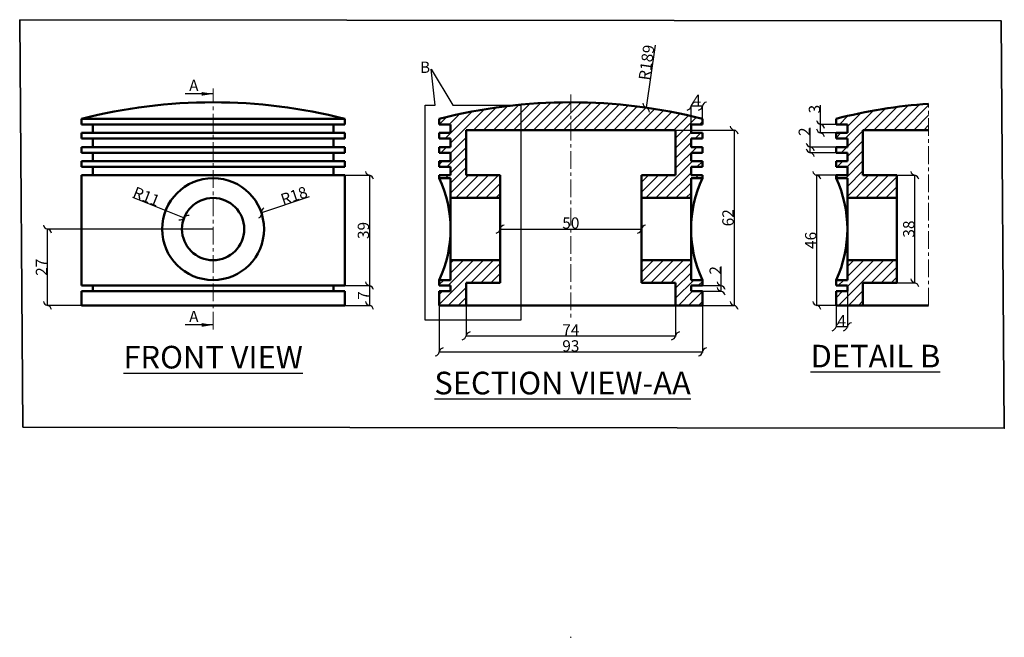
# Model space of a CAD drawing. Units: millimetres. Extents: x 25 to 373, y -30 to 188.
import ezdxf

# ---------------------------------------------------------------- set-up
doc = ezdxf.new("R2010")
doc.units = ezdxf.units.MM
doc.header["$MEASUREMENT"] = 0
doc.linetypes.add('CENTER', pattern=[2, 1.25, -0.25, 0.25, -0.25])
for name, color, linetype, lineweight in [('M-CNTR', 1, 'CENTER', 18), ('M-DIMS', 2, 'Continuous', 25), ('M-HATC', 8, 'Continuous', 18), ('M-OUTL', 7, 'Continuous', 50), ('M-SYMB', 4, 'Continuous', 25), ('M-TEXT', 7, 'Continuous', 25), ('M-TTLB', 7, 'Continuous', 35)]:
    doc.layers.add(name, color=color, linetype=linetype, lineweight=lineweight)
doc.styles.get("Standard").update_dxf_attribs({"font": 'arial.ttf'})
doc.dimstyles.get("Standard").update_dxf_attribs({"dimtxt": 4, "dimasz": 4, "dimexe": 0.18, "dimexo": 0.0625, "dimgap": 0.09, "dimtad": 1, "dimdec": 0, "dimzin": 0, "dimdsep": 46, "dimtxsty": 'Standard', "dimblk": 'INTEGRAL', "dimcen": 0.09, "dimclre": 251, "dimadec": 0, "dimazin": 0, "dimtfac": 1, "dimtdec": 0, "dimtofl": 0, "dimtmove": 0, "dimatfit": 3, "dimfxl": 1, "dimtolj": 1, "dimtzin": 0, "dimarcsym": 0})
pattern_1 = [(45, (-84.6506, -72.2626), (-1.767767, 1.767767), [])]

# ---------------------------------------------------------------- blocks, each defined once
blk = doc.blocks.new('_Integral')
at = {"color": 0, "linetype": 'ByBlock', "lineweight": -2}
for centre, start, end in [((0.445, -0.091), 102, 168), ((-0.445, 0.091), 282, 348)]:
    blk.add_arc(centre, 0.454, start, end, dxfattribs=at)
blk = doc.blocks.new('*D2')
at = {"layer": 'Defpoints', "color": 0, "transparency": 16777216}
for p in [(308.49, 150.79), (313.98, 150.79), (313.98, 147.79)]:
    blk.add_point(p, dxfattribs=at)
at = {"layer": 'M-DIMS', "color": 0, "lineweight": -2, "transparency": 16777216}
for p, q in [((308.49, 150.79), (308.49, 157.59)), ((313.92, 150.79), (308.31, 150.79)), ((308.49, 147.79), (308.49, 150.79)), ((313.92, 147.79), (308.31, 147.79))]:
    blk.add_line(p, q, dxfattribs=at)
at = {"layer": 'M-DIMS', "color": 0, "lineweight": -2, "transparency": 16777216, "xscale": 4, "yscale": 4, "zscale": 4}
for p, rotation in [((308.49, 150.79), 90), ((308.49, 147.79), 270)]:
    blk.add_blockref('_Integral', p, dxfattribs=dict(at, rotation=rotation))
at = {"layer": 'M-DIMS', "color": 0, "transparency": 16777216, "insert": (306.36, 156.19), "char_height": 4, "attachment_point": 5, "rotation": 90}
blk.add_mtext('\\A1;3', dxfattribs=at)
blk = doc.blocks.new('*D3')
at = {"layer": 'Defpoints', "color": 0, "transparency": 16777216}
for p in [(313.98, 142.79), (304.86, 140.79), (313.98, 140.79)]:
    blk.add_point(p, dxfattribs=at)
at = {"layer": 'M-DIMS', "color": 0, "lineweight": -2, "transparency": 16777216}
for p, q in [((304.86, 142.79), (304.86, 149.62)), ((313.92, 142.79), (304.68, 142.79)), ((304.86, 140.79), (304.86, 142.79)), ((313.92, 140.79), (304.68, 140.79))]:
    blk.add_line(p, q, dxfattribs=at)
at = {"layer": 'M-DIMS', "color": 0, "lineweight": -2, "transparency": 16777216, "xscale": 4, "yscale": 4, "zscale": 4}
for p, rotation in [((304.86, 142.79), 90), ((304.86, 140.79), 270)]:
    blk.add_blockref('_Integral', p, dxfattribs=dict(at, rotation=rotation))
at = {"layer": 'M-DIMS', "color": 0, "transparency": 16777216, "insert": (302.76, 148.2), "char_height": 4, "attachment_point": 5, "rotation": 90}
blk.add_mtext('\\A1;2', dxfattribs=at)
blk = doc.blocks.new('*D4')
at = {"layer": 'Defpoints', "color": 0, "transparency": 16777216}
for p in [(307.16, 132.79), (313.98, 132.79), (313.98, 86.79)]:
    blk.add_point(p, dxfattribs=at)
at = {"layer": 'M-DIMS', "color": 0, "lineweight": -2, "transparency": 16777216}
for p, q in [((313.92, 132.79), (306.98, 132.79)), ((307.16, 86.79), (307.16, 132.79)), ((313.92, 86.79), (306.98, 86.79))]:
    blk.add_line(p, q, dxfattribs=at)
at = {"layer": 'M-DIMS', "color": 0, "lineweight": -2, "transparency": 16777216, "xscale": 4, "yscale": 4, "zscale": 4}
for p, rotation in [((307.16, 132.79), 90), ((307.16, 86.79), 270)]:
    blk.add_blockref('_Integral', p, dxfattribs=dict(at, rotation=rotation))
at = {"layer": 'M-DIMS', "color": 0, "transparency": 16777216, "insert": (305.03, 109.79), "char_height": 4, "attachment_point": 5, "rotation": 90}
blk.add_mtext('\\A1;46', dxfattribs=at)
blk = doc.blocks.new('*D5')
at = {"layer": 'Defpoints', "color": 0, "transparency": 16777216}
for p in [(317.98, 91.79), (313.98, 86.79), (313.98, 79.29)]:
    blk.add_point(p, dxfattribs=at)
at = {"layer": 'M-DIMS', "color": 0, "lineweight": -2, "transparency": 16777216}
for p, q in [((317.98, 91.73), (317.98, 79.11)), ((313.98, 86.73), (313.98, 79.11)), ((317.98, 79.29), (313.98, 79.29))]:
    blk.add_line(p, q, dxfattribs=at)
at = {"layer": 'M-DIMS', "color": 0, "lineweight": -2, "transparency": 16777216, "xscale": 4, "yscale": 4, "zscale": 4, "rotation": 180}
blk.add_blockref('_Integral', (313.98, 79.29), dxfattribs=at)
at = {"layer": 'M-DIMS', "color": 0, "lineweight": -2, "transparency": 16777216, "xscale": 4, "yscale": 4, "zscale": 4}
blk.add_blockref('_Integral', (317.98, 79.29), dxfattribs=at)
at = {"layer": 'M-DIMS', "color": 0, "transparency": 16777216, "insert": (315.98, 81.38), "char_height": 4, "attachment_point": 5}
blk.add_mtext('\\A1;4', dxfattribs=at)
blk = doc.blocks.new('*D6')
at = {"layer": 'Defpoints', "color": 0, "transparency": 16777216}
for p in [(335.48, 132.79), (341.81, 132.79), (335.48, 94.79)]:
    blk.add_point(p, dxfattribs=at)
at = {"layer": 'M-DIMS', "color": 0, "lineweight": -2, "transparency": 16777216}
for p, q in [((335.54, 132.79), (341.99, 132.79)), ((341.81, 94.79), (341.81, 132.79)), ((335.54, 94.79), (341.99, 94.79))]:
    blk.add_line(p, q, dxfattribs=at)
at = {"layer": 'M-DIMS', "color": 0, "lineweight": -2, "transparency": 16777216, "xscale": 4, "yscale": 4, "zscale": 4}
for p, rotation in [((341.81, 132.79), 90), ((341.81, 94.79), 270)]:
    blk.add_blockref('_Integral', p, dxfattribs=dict(at, rotation=rotation))
at = {"layer": 'M-DIMS', "color": 0, "transparency": 16777216, "insert": (339.67, 113.79), "char_height": 4, "attachment_point": 5, "rotation": 90}
blk.add_mtext('\\A1;38', dxfattribs=at)
blk = doc.blocks.new('*D7')
at = {"layer": 'Defpoints', "color": 0, "transparency": 16777216}
for p in [(246.9, 156.71), (220.26, -30.4)]:
    blk.add_point(p, dxfattribs=at)
at = {"layer": 'M-DIMS', "color": 0, "lineweight": -2, "transparency": 16777216}
for p, q in [((250.04, 178.74), (246.9, 156.71)), ((220.17, -30.4), (220.35, -30.4)), ((220.26, -30.49), (220.26, -30.31))]:
    blk.add_line(p, q, dxfattribs=at)
at = {"layer": 'M-DIMS', "color": 0, "lineweight": -2, "transparency": 16777216, "xscale": 4, "yscale": 4, "zscale": 4, "rotation": 261.8951783381606}
blk.add_blockref('_Integral', (246.9, 156.71), dxfattribs=at)
at = {"layer": 'M-DIMS', "color": 0, "transparency": 16777216, "insert": (247.02, 172.67), "char_height": 4, "attachment_point": 5, "rotation": 81.8952}
blk.add_mtext('\\A1;R189', dxfattribs=at)
blk = doc.blocks.new('*D8')
at = {"layer": 'Defpoints', "color": 0, "transparency": 16777216}
for p in [(262.76, 157.24), (262.76, 150.79), (266.76, 150.79)]:
    blk.add_point(p, dxfattribs=at)
at = {"layer": 'M-DIMS', "color": 0, "lineweight": -2, "transparency": 16777216}
for p, q in [((262.76, 150.85), (262.76, 157.42)), ((266.76, 157.24), (262.76, 157.24)), ((266.76, 150.85), (266.76, 157.42))]:
    blk.add_line(p, q, dxfattribs=at)
at = {"layer": 'M-DIMS', "color": 0, "lineweight": -2, "transparency": 16777216, "xscale": 4, "yscale": 4, "zscale": 4, "rotation": 180}
blk.add_blockref('_Integral', (262.76, 157.24), dxfattribs=at)
at = {"layer": 'M-DIMS', "color": 0, "lineweight": -2, "transparency": 16777216, "xscale": 4, "yscale": 4, "zscale": 4}
blk.add_blockref('_Integral', (266.76, 157.24), dxfattribs=at)
at = {"layer": 'M-DIMS', "color": 0, "transparency": 16777216, "insert": (264.76, 159.33), "char_height": 4, "attachment_point": 5}
blk.add_mtext('\\A1;4', dxfattribs=at)
blk = doc.blocks.new('*D9')
at = {"layer": 'Defpoints', "color": 0, "transparency": 16777216}
for p in [(257.26, 148.79), (266.76, 86.79), (277.92, 86.79)]:
    blk.add_point(p, dxfattribs=at)
at = {"layer": 'M-DIMS', "color": 0, "lineweight": -2, "transparency": 16777216}
for p, q in [((257.32, 148.79), (278.1, 148.79)), ((277.92, 148.79), (277.92, 86.79)), ((266.82, 86.79), (278.1, 86.79))]:
    blk.add_line(p, q, dxfattribs=at)
at = {"layer": 'M-DIMS', "color": 0, "lineweight": -2, "transparency": 16777216, "xscale": 4, "yscale": 4, "zscale": 4}
for p, rotation in [((277.92, 148.79), 90), ((277.92, 86.79), 270)]:
    blk.add_blockref('_Integral', p, dxfattribs=dict(at, rotation=rotation))
at = {"layer": 'M-DIMS', "color": 0, "transparency": 16777216, "insert": (275.79, 117.79), "char_height": 4, "attachment_point": 5, "rotation": 90}
blk.add_mtext('\\A1;62', dxfattribs=at)
blk = doc.blocks.new('*D10')
at = {"layer": 'Defpoints', "color": 0, "transparency": 16777216}
for p in [(266.76, 93.79), (266.76, 91.79), (273.36, 93.79)]:
    blk.add_point(p, dxfattribs=at)
at = {"layer": 'M-DIMS', "color": 0, "lineweight": -2, "transparency": 16777216}
for p, q in [((273.36, 93.79), (273.36, 100.62)), ((266.82, 93.79), (273.54, 93.79)), ((266.82, 91.79), (273.54, 91.79)), ((273.36, 91.79), (273.36, 93.79))]:
    blk.add_line(p, q, dxfattribs=at)
at = {"layer": 'M-DIMS', "color": 0, "lineweight": -2, "transparency": 16777216, "xscale": 4, "yscale": 4, "zscale": 4}
for p, rotation in [((273.36, 93.79), 90), ((273.36, 91.79), 270)]:
    blk.add_blockref('_Integral', p, dxfattribs=dict(at, rotation=rotation))
at = {"layer": 'M-DIMS', "color": 0, "transparency": 16777216, "insert": (271.26, 99.2), "char_height": 4, "attachment_point": 5, "rotation": 90}
blk.add_mtext('\\A1;2', dxfattribs=at)
blk = doc.blocks.new('*D11')
at = {"layer": 'Defpoints', "color": 0, "transparency": 16777216}
for p in [(195.26, 113.79), (245.26, 113.79), (245.26, 113.79)]:
    blk.add_point(p, dxfattribs=at)
at = {"layer": 'M-DIMS', "color": 0, "lineweight": -2, "transparency": 16777216}
for p, q in [((195.26, 113.85), (195.26, 113.97)), ((195.26, 113.79), (245.26, 113.79)), ((245.26, 113.85), (245.26, 113.97))]:
    blk.add_line(p, q, dxfattribs=at)
at = {"layer": 'M-DIMS', "color": 0, "lineweight": -2, "transparency": 16777216, "xscale": 4, "yscale": 4, "zscale": 4, "rotation": 180}
blk.add_blockref('_Integral', (195.26, 113.79), dxfattribs=at)
at = {"layer": 'M-DIMS', "color": 0, "lineweight": -2, "transparency": 16777216, "xscale": 4, "yscale": 4, "zscale": 4}
blk.add_blockref('_Integral', (245.26, 113.79), dxfattribs=at)
at = {"layer": 'M-DIMS', "color": 0, "transparency": 16777216, "insert": (220.26, 115.92), "char_height": 4, "attachment_point": 5}
blk.add_mtext('\\A1;50', dxfattribs=at)
blk = doc.blocks.new('*D12')
at = {"layer": 'Defpoints', "color": 0, "transparency": 16777216}
for p in [(173.76, 86.79), (266.76, 86.79), (266.76, 70.37)]:
    blk.add_point(p, dxfattribs=at)
at = {"layer": 'M-DIMS', "color": 0, "lineweight": -2, "transparency": 16777216}
for p, q in [((173.76, 86.73), (173.76, 70.19)), ((266.76, 86.73), (266.76, 70.19)), ((173.76, 70.37), (266.76, 70.37))]:
    blk.add_line(p, q, dxfattribs=at)
at = {"layer": 'M-DIMS', "color": 0, "lineweight": -2, "transparency": 16777216, "xscale": 4, "yscale": 4, "zscale": 4, "rotation": 180}
blk.add_blockref('_Integral', (173.76, 70.37), dxfattribs=at)
at = {"layer": 'M-DIMS', "color": 0, "lineweight": -2, "transparency": 16777216, "xscale": 4, "yscale": 4, "zscale": 4}
blk.add_blockref('_Integral', (266.76, 70.37), dxfattribs=at)
at = {"layer": 'M-DIMS', "color": 0, "transparency": 16777216, "insert": (220.26, 72.5), "char_height": 4, "attachment_point": 5}
blk.add_mtext('\\A1;93', dxfattribs=at)
blk = doc.blocks.new('*D13')
at = {"layer": 'Defpoints', "color": 0, "transparency": 16777216}
for p in [(183.26, 86.79), (257.26, 86.79), (257.26, 76.06)]:
    blk.add_point(p, dxfattribs=at)
at = {"layer": 'M-DIMS', "color": 0, "lineweight": -2, "transparency": 16777216}
for p, q in [((183.26, 86.73), (183.26, 75.88)), ((257.26, 86.73), (257.26, 75.88)), ((183.26, 76.06), (257.26, 76.06))]:
    blk.add_line(p, q, dxfattribs=at)
at = {"layer": 'M-DIMS', "color": 0, "lineweight": -2, "transparency": 16777216, "xscale": 4, "yscale": 4, "zscale": 4, "rotation": 180}
blk.add_blockref('_Integral', (183.26, 76.06), dxfattribs=at)
at = {"layer": 'M-DIMS', "color": 0, "lineweight": -2, "transparency": 16777216, "xscale": 4, "yscale": 4, "zscale": 4}
blk.add_blockref('_Integral', (257.26, 76.06), dxfattribs=at)
at = {"layer": 'M-DIMS', "color": 0, "transparency": 16777216, "insert": (220.26, 78.15), "char_height": 4, "attachment_point": 5}
blk.add_mtext('\\A1;74', dxfattribs=at)
blk = doc.blocks.new('*D14')
at = {"layer": 'Defpoints', "color": 0, "transparency": 16777216}
for p in [(140.34, 132.79), (140.34, 93.79), (149.09, 93.79)]:
    blk.add_point(p, dxfattribs=at)
at = {"layer": 'M-DIMS', "color": 0, "lineweight": -2, "transparency": 16777216}
for p, q in [((140.4, 132.79), (149.27, 132.79)), ((149.09, 132.79), (149.09, 93.79)), ((140.4, 93.79), (149.27, 93.79))]:
    blk.add_line(p, q, dxfattribs=at)
at = {"layer": 'M-DIMS', "color": 0, "lineweight": -2, "transparency": 16777216, "xscale": 4, "yscale": 4, "zscale": 4}
for p, rotation in [((149.09, 132.79), 90), ((149.09, 93.79), 270)]:
    blk.add_blockref('_Integral', p, dxfattribs=dict(at, rotation=rotation))
at = {"layer": 'M-DIMS', "color": 0, "transparency": 16777216, "insert": (146.95, 113.29), "char_height": 4, "attachment_point": 5, "rotation": 90}
blk.add_mtext('\\A1;39', dxfattribs=at)
blk = doc.blocks.new('*D15')
at = {"layer": 'Defpoints', "color": 0, "transparency": 16777216}
for p in [(140.34, 93.79), (140.34, 86.79), (149.08, 86.79)]:
    blk.add_point(p, dxfattribs=at)
at = {"layer": 'M-DIMS', "color": 0, "lineweight": -2, "transparency": 16777216}
for p, q in [((140.4, 93.79), (149.26, 93.79)), ((149.08, 93.79), (149.08, 86.79)), ((140.4, 86.79), (149.26, 86.79))]:
    blk.add_line(p, q, dxfattribs=at)
at = {"layer": 'M-DIMS', "color": 0, "lineweight": -2, "transparency": 16777216, "xscale": 4, "yscale": 4, "zscale": 4}
for p, rotation in [((149.08, 93.79), 90), ((149.08, 86.79), 270)]:
    blk.add_blockref('_Integral', p, dxfattribs=dict(at, rotation=rotation))
at = {"layer": 'M-DIMS', "color": 0, "transparency": 16777216, "insert": (146.99, 90.29), "char_height": 4, "attachment_point": 5, "rotation": 90}
blk.add_mtext('\\A1;7', dxfattribs=at)
blk = doc.blocks.new('*D16')
at = {"layer": 'Defpoints', "color": 0, "transparency": 16777216}
for p in [(35.29, 113.79), (93.84, 113.79), (47.34, 86.79)]:
    blk.add_point(p, dxfattribs=at)
at = {"layer": 'M-DIMS', "color": 0, "lineweight": -2, "transparency": 16777216}
for p, q in [((93.77, 113.79), (35.11, 113.79)), ((35.29, 86.79), (35.29, 113.79)), ((47.27, 86.79), (35.11, 86.79))]:
    blk.add_line(p, q, dxfattribs=at)
at = {"layer": 'M-DIMS', "color": 0, "lineweight": -2, "transparency": 16777216, "xscale": 4, "yscale": 4, "zscale": 4}
for p, rotation in [((35.29, 113.79), 90), ((35.29, 86.79), 270)]:
    blk.add_blockref('_Integral', p, dxfattribs=dict(at, rotation=rotation))
at = {"layer": 'M-DIMS', "color": 0, "transparency": 16777216, "insert": (33.19, 100.29), "char_height": 4, "attachment_point": 5, "rotation": 90}
blk.add_mtext('\\A1;27', dxfattribs=at)
blk = doc.blocks.new('*D17')
at = {"layer": 'Defpoints', "color": 0, "transparency": 16777216}
for p in [(110.91, 119.5), (93.84, 113.79)]:
    blk.add_point(p, dxfattribs=at)
at = {"layer": 'M-DIMS', "color": 0, "lineweight": -2, "transparency": 16777216}
for p, q in [((127.74, 125.13), (110.91, 119.5)), ((93.75, 113.79), (93.93, 113.79)), ((93.84, 113.7), (93.84, 113.88))]:
    blk.add_line(p, q, dxfattribs=at)
at = {"layer": 'M-DIMS', "color": 0, "lineweight": -2, "transparency": 16777216, "xscale": 4, "yscale": 4, "zscale": 4, "rotation": 198.4934261672006}
blk.add_blockref('_Integral', (110.91, 119.5), dxfattribs=at)
at = {"layer": 'M-DIMS', "color": 0, "transparency": 16777216, "insert": (122.44, 125.6), "char_height": 4, "attachment_point": 5, "rotation": 18.4934}
blk.add_mtext('\\A1;R18', dxfattribs=at)
blk = doc.blocks.new('*D18')
at = {"layer": 'Defpoints', "color": 0, "transparency": 16777216}
for p in [(83.6, 117.82), (93.84, 113.79)]:
    blk.add_point(p, dxfattribs=at)
at = {"layer": 'M-DIMS', "color": 0, "lineweight": -2, "transparency": 16777216}
for p, q in [((65.35, 125.01), (83.6, 117.82)), ((93.75, 113.79), (93.93, 113.79)), ((93.84, 113.7), (93.84, 113.88))]:
    blk.add_line(p, q, dxfattribs=at)
at = {"layer": 'M-DIMS', "color": 0, "lineweight": -2, "transparency": 16777216, "xscale": 4, "yscale": 4, "zscale": 4, "rotation": 338.4984273630489}
blk.add_blockref('_Integral', (83.6, 117.82), dxfattribs=at)
at = {"layer": 'M-DIMS', "color": 0, "transparency": 16777216, "insert": (70.28, 125.32), "char_height": 4, "attachment_point": 5, "rotation": 338.4984}
blk.add_mtext('\\A1;R11', dxfattribs=at)

msp = doc.modelspace()

# ---------------------------------------------------------------- hatches: boundary and pattern name
at = {"layer": 'M-HATC'}
h = msp.add_hatch(dxfattribs=at)
h.set_pattern_fill('ANSI31', color=256, scale=20)
h.set_pattern_definition(pattern_1)
h.paths.add_polyline_path([(195.26, 132.79), (183.26, 132.79), (183.26, 148.79), (220.26, 148.79), (220.26, 158.6, 0.062226), (173.76, 152.79), (173.76, 150.79), (177.76, 150.79), (177.76, 147.79), (173.76, 147.79), (173.76, 145.79), (177.76, 145.79), (177.76, 142.79), (173.76, 142.79), (173.76, 140.79), (177.76, 140.79), (177.76, 137.79), (173.76, 137.79), (173.76, 135.79), (177.76, 135.79), (177.76, 132.79), (173.76, 132.79), (173.76, 131.79), (177.76, 131.79), (177.76, 124.79), (195.26, 124.79)])
h.paths.add_polyline_path([(266.76, 152.79, 0.062226), (220.26, 158.6), (220.26, 148.79), (257.26, 148.79), (257.26, 132.79), (245.26, 132.79), (245.26, 124.79), (262.76, 124.79), (262.76, 131.79), (266.76, 131.79), (266.76, 132.79), (262.76, 132.79), (262.76, 135.79), (266.76, 135.79), (266.76, 137.79), (262.76, 137.79), (262.76, 140.79), (266.76, 140.79), (266.76, 142.79), (262.76, 142.79), (262.76, 145.79), (266.76, 145.79), (266.76, 147.79), (262.76, 147.79), (262.76, 150.79), (266.76, 150.79)])
h.paths.add_polyline_path([(262.76, 102.79), (245.26, 102.79), (245.26, 94.79), (257.26, 94.79), (257.26, 86.79), (266.76, 86.79), (266.76, 91.79), (262.76, 91.79), (262.76, 93.79), (266.76, 93.79), (266.76, 95.79), (262.76, 95.79)])
h.paths.add_polyline_path([(195.26, 102.79), (177.76, 102.79), (177.76, 95.79), (173.76, 95.79), (173.76, 93.79), (177.76, 93.79), (177.76, 91.79), (173.76, 91.79), (173.76, 86.79), (183.26, 86.79), (183.26, 94.79), (195.26, 94.79)])
h = msp.add_hatch(dxfattribs=at)
h.set_pattern_fill('ANSI31', color=256, scale=20)
h.set_pattern_definition(pattern_1)
h.paths.add_polyline_path([(317.98, 102.79), (317.98, 95.79), (313.98, 95.79), (313.98, 93.79), (317.98, 93.79), (317.98, 91.79), (313.98, 91.79), (313.98, 86.79), (323.48, 86.79), (323.48, 94.79), (335.48, 94.79), (335.48, 102.79)])
h.paths.add_polyline_path([(323.48, 132.79), (323.48, 148.79), (346.69, 148.79), (346.69, 158.09, 0.043924), (313.98, 152.79), (313.98, 150.79), (317.98, 150.79), (317.98, 147.79), (313.98, 147.79), (313.98, 145.79), (317.98, 145.79), (317.98, 142.79), (313.98, 142.79), (313.98, 140.79), (317.98, 140.79), (317.98, 137.79), (313.98, 137.79), (313.98, 135.79), (317.98, 135.79), (317.98, 132.79), (313.98, 132.79), (313.98, 131.79), (317.98, 131.79), (317.98, 124.79), (335.48, 124.79), (335.48, 132.79)])

# ---------------------------------------------------------------- linework, layer by layer
at = {"layer": 'M-CNTR', "ltscale": 5}
for p, q in [((93.84, 78.31), (93.84, 163.48)), ((220.26, 161.34), (220.26, 82.21)), ((346.69, 86.79), (346.69, 158.09))]:
    msp.add_line(p, q, dxfattribs=at)
at = {"layer": 'M-OUTL'}
for p, q in [((47.34, 150.79), (47.34, 152.79)), ((47.34, 152.79), (140.34, 152.79)), ((140.34, 150.79), (47.34, 150.79)), ((51.34, 147.79), (51.34, 150.79)), ((51.34, 150.79), (51.34, 147.79)), ((136.34, 150.79), (136.34, 147.79)), ((140.34, 150.79), (140.34, 152.79)), ((173.76, 150.79), (173.76, 152.79)), ((177.76, 150.79), (173.76, 150.79)), ((177.76, 147.79), (177.76, 150.79)), ((262.76, 147.79), (262.76, 150.79)), ((262.76, 150.79), (266.76, 150.79)), ((266.76, 150.79), (266.76, 152.79)), ((313.98, 150.79), (313.98, 152.79)), ((317.98, 150.79), (313.98, 150.79)), ((317.98, 147.79), (317.98, 150.79)), ((47.34, 145.79), (47.34, 147.79)), ((47.34, 147.79), (140.34, 147.79)), ((140.34, 145.79), (140.34, 147.79)), ((173.76, 145.79), (173.76, 147.79)), ((173.76, 147.79), (177.76, 147.79)), ((183.26, 148.79), (257.26, 148.79)), ((183.26, 132.79), (183.26, 148.79)), ((257.26, 148.79), (257.26, 132.79)), ((266.76, 147.79), (262.76, 147.79)), ((266.76, 145.79), (266.76, 147.79)), ((313.98, 145.79), (313.98, 147.79)), ((313.98, 147.79), (317.98, 147.79)), ((323.48, 148.79), (346.69, 148.79)), ((323.48, 132.79), (323.48, 148.79)), ((140.34, 145.79), (47.34, 145.79)), ((47.34, 140.79), (47.34, 142.79)), ((47.34, 142.79), (140.34, 142.79)), ((51.34, 142.79), (51.34, 145.79)), ((51.34, 145.79), (51.34, 142.79)), ((136.34, 145.79), (136.34, 142.79)), ((140.34, 140.79), (140.34, 142.79)), ((177.76, 145.79), (173.76, 145.79)), ((173.76, 140.79), (173.76, 142.79)), ((173.76, 142.79), (177.76, 142.79)), ((177.76, 142.79), (177.76, 145.79)), ((262.76, 142.79), (262.76, 145.79)), ((262.76, 145.79), (266.76, 145.79)), ((266.76, 142.79), (262.76, 142.79)), ((266.76, 140.79), (266.76, 142.79)), ((317.98, 145.79), (313.98, 145.79)), ((313.98, 140.79), (313.98, 142.79)), ((313.98, 142.79), (317.98, 142.79)), ((317.98, 142.79), (317.98, 145.79)), ((140.34, 140.79), (47.34, 140.79)), ((51.34, 137.79), (51.34, 140.79)), ((51.34, 140.79), (51.34, 137.79)), ((136.34, 140.79), (136.34, 137.79)), ((177.76, 140.79), (173.76, 140.79)), ((177.76, 137.79), (177.76, 140.79)), ((262.76, 137.79), (262.76, 140.79)), ((262.76, 140.79), (266.76, 140.79)), ((317.98, 140.79), (313.98, 140.79)), ((317.98, 137.79), (317.98, 140.79)), ((47.34, 135.79), (47.34, 137.79)), ((47.34, 137.79), (140.34, 137.79)), ((140.34, 135.79), (47.34, 135.79)), ((51.34, 133.79), (51.34, 135.79)), ((51.34, 135.79), (51.34, 132.79)), ((136.34, 135.79), (136.34, 132.79)), ((140.34, 135.79), (140.34, 137.79)), ((173.76, 135.79), (173.76, 137.79)), ((173.76, 137.79), (177.76, 137.79)), ((177.76, 135.79), (173.76, 135.79)), ((177.76, 132.79), (177.76, 135.79)), ((266.76, 137.79), (262.76, 137.79)), ((262.76, 132.79), (262.76, 135.79)), ((262.76, 135.79), (266.76, 135.79)), ((266.76, 135.79), (266.76, 137.79)), ((313.98, 135.79), (313.98, 137.79)), ((313.98, 137.79), (317.98, 137.79)), ((317.98, 135.79), (313.98, 135.79)), ((317.98, 132.79), (317.98, 135.79)), ((47.34, 93.79), (47.34, 132.79)), ((47.34, 132.79), (140.34, 132.79)), ((140.34, 93.79), (140.34, 132.79)), ((173.76, 131.79), (173.76, 132.79)), ((173.76, 132.79), (177.76, 132.79)), ((183.26, 132.79), (195.26, 132.79)), ((195.26, 94.79), (195.26, 132.79)), ((245.26, 132.79), (257.26, 132.79)), ((245.26, 94.79), (245.26, 132.79)), ((266.76, 132.79), (262.76, 132.79)), ((266.76, 131.79), (266.76, 132.79)), ((313.98, 131.79), (313.98, 132.79)), ((313.98, 132.79), (317.98, 132.79)), ((323.48, 132.79), (335.48, 132.79)), ((335.48, 94.79), (335.48, 132.79)), ((177.76, 131.79), (173.76, 131.79)), ((177.76, 95.79), (177.76, 131.79)), ((262.76, 95.79), (262.76, 131.79)), ((262.76, 131.79), (266.76, 131.79)), ((317.98, 131.79), (313.98, 131.79)), ((317.98, 95.79), (317.98, 131.79)), ((177.76, 124.79), (195.26, 124.79)), ((245.26, 124.79), (262.76, 124.79)), ((317.98, 124.79), (335.48, 124.79)), ((177.76, 102.79), (195.26, 102.79)), ((245.26, 102.79), (262.76, 102.79)), ((317.98, 102.79), (335.48, 102.79)), ((173.76, 93.79), (173.76, 95.79)), ((173.76, 95.79), (177.76, 95.79)), ((183.26, 94.79), (183.26, 86.79)), ((183.26, 94.79), (195.26, 94.79)), ((245.26, 94.79), (257.26, 94.79)), ((257.26, 94.79), (257.26, 86.79)), ((266.76, 95.79), (262.76, 95.79)), ((266.76, 93.79), (266.76, 95.79)), ((313.98, 93.79), (313.98, 95.79)), ((313.98, 95.79), (317.98, 95.79)), ((323.48, 94.79), (323.48, 86.79)), ((323.48, 94.79), (335.48, 94.79)), ((47.34, 93.79), (140.34, 93.79)), ((47.34, 91.79), (140.34, 91.79)), ((47.34, 86.79), (47.34, 91.79)), ((51.34, 91.79), (51.34, 93.79)), ((136.34, 91.79), (136.34, 93.79)), ((140.34, 91.79), (140.34, 86.79)), ((177.76, 93.79), (173.76, 93.79)), ((173.76, 86.79), (173.76, 91.79)), ((173.76, 91.79), (177.76, 91.79)), ((177.76, 91.79), (177.76, 93.79)), ((262.76, 91.79), (262.76, 93.79)), ((262.76, 93.79), (266.76, 93.79)), ((266.76, 91.79), (262.76, 91.79)), ((266.76, 86.79), (266.76, 91.79)), ((317.98, 93.79), (313.98, 93.79)), ((313.98, 86.79), (313.98, 91.79)), ((313.98, 91.79), (317.98, 91.79)), ((317.98, 91.79), (317.98, 93.79)), ((47.34, 86.79), (140.34, 86.79)), ((173.76, 86.79), (266.76, 86.79)), ((313.98, 86.79), (346.69, 86.79))]:
    msp.add_line(p, q, dxfattribs=at)
for radius in [18, 11]:
    msp.add_circle((93.84, 113.79), radius, dxfattribs=at)
for centre, radius, start, end in [((93.84, -30.4), 189, 75.7572, 104.2428), ((220.26, -30.4), 189, 75.7572, 104.2428), ((360.48, -30.4), 189, 94.1825, 104.2428), ((135.26, 113.79), 42.5, 334.9424, 25.0576), ((305.26, 113.79), 42.5, 154.9424, 205.0576), ((275.48, 113.79), 42.5, 334.9424, 25.0576)]:
    msp.add_arc(centre, radius, start, end, dxfattribs=at)
at = {"layer": 'M-SYMB'}
for p, q in [((172.28, 157.61), (170.86, 170.31)), ((170.86, 170.31), (178.5, 157.61))]:
    msp.add_line(p, q, dxfattribs=at)
msp.add_lwpolyline([(178.5, 157.61), (202.58, 157.61), (202.58, 81.63), (168.8, 81.63), (168.8, 157.61), (172.28, 157.61)], dxfattribs=at)
at = {"layer": 'M-TTLB'}
msp.add_lwpolyline([(25.49, 187.79), (372.32, 187.4), (373.44, 43.4), (26.61, 43.79)], close=True, dxfattribs=at)

# ---------------------------------------------------------------- texts
at = {"layer": 'M-TEXT', "char_height": 4, "attachment_point": 5}
for s, insert in [('\\A1;B', (168.74, 170.98)), ('\\A1;A', (87.03, 164.56)), ('\\A1;A', (87.03, 82.89))]:
    msp.add_mtext(s, dxfattribs=dict(at, insert=insert))
at = {"layer": 'M-TEXT', "char_height": 8, "attachment_point": 1}
for s, width, insert in [('{\\LFRONT VIEW}', 89.221, (62.15, 72.52)), ('{\\LDETAIL B}', 89.221, (304.98, 72.89)), ('{\\LSECTION VIEW-AA}', 124.3685, (172.03, 63.37))]:
    msp.add_mtext_dynamic_manual_height_columns(s, width=width, gutter_width=1, heights=[0], dxfattribs=dict(at, insert=insert))

# ---------------------------------------------------------------- dimensions: what is measured, and where the dimension line sits
at = {"layer": 'M-DIMS'}
for center, mpoint, picture, middle in [((220.26, -30.4), (246.9, 156.71), '*D7', (249.14, 172.37)), ((93.84, 113.79), (83.6, 117.82), '*D18', (69.52, 123.37))]:
    dim = msp.add_radius_dim(center=center, mpoint=mpoint, dimstyle='Standard', override={"dimclrd": 0, "dimclre": 0, "dimclrt": 0}, dxfattribs=at)
    dim.commit()
    dim.dimension.update_dxf_attribs({"geometry": picture, "text_midpoint": middle, "dimtype": 164})
for base, p1, p2, picture, middle in [((262.76, 157.24), (266.76, 150.79), (262.76, 150.79), '*D8', (264.76, 159.33)), ((245.26, 113.79), (195.26, 113.79), (245.26, 113.79), '*D11', (220.26, 115.92)), ((313.98, 79.29), (317.98, 91.79), (313.98, 86.79), '*D5', (315.98, 81.38)), ((266.76, 70.37), (173.76, 86.79), (266.76, 86.79), '*D12', (220.26, 72.5)), ((257.26, 76.06), (183.26, 86.79), (257.26, 86.79), '*D13', (220.26, 78.15))]:
    dim = msp.add_linear_dim(base=base, p1=p1, p2=p2, dimstyle='Standard', override={"dimclrd": 0, "dimclre": 0, "dimclrt": 0}, dxfattribs=at)
    dim.commit()
    dim.dimension.update_dxf_attribs({"geometry": picture, "text_midpoint": middle})
for base, p1, p2, picture, middle in [((308.49, 150.79), (313.98, 147.79), (313.98, 150.79), '*D2', (308.49, 156.19)), ((304.86, 140.79), (313.98, 142.79), (313.98, 140.79), '*D3', (304.86, 148.2))]:
    dim = msp.add_linear_dim(base=base, p1=p1, p2=p2, angle=90, dimstyle='Standard', override={"dimclrd": 0, "dimclre": 0, "dimclrt": 0}, dxfattribs=at)
    dim.commit()
    dim.dimension.update_dxf_attribs({"geometry": picture, "text_midpoint": middle, "dimtype": 160})
for base, p1, p2, picture, middle in [((277.92, 86.79), (257.26, 148.79), (266.76, 86.79), '*D9', (275.79, 117.79)), ((149.09, 93.79), (140.34, 132.79), (140.34, 93.79), '*D14', (146.95, 113.29)), ((307.16, 132.79), (313.98, 86.79), (313.98, 132.79), '*D4', (305.03, 109.79)), ((341.81, 132.79), (335.48, 94.79), (335.48, 132.79), '*D6', (339.67, 113.79)), ((35.29, 113.79), (47.34, 86.79), (93.84, 113.79), '*D16', (33.19, 100.29)), ((273.36, 93.79), (266.76, 91.79), (266.76, 93.79), '*D10', (271.26, 99.2)), ((149.08, 86.79), (140.34, 93.79), (140.34, 86.79), '*D15', (146.99, 90.29))]:
    dim = msp.add_linear_dim(base=base, p1=p1, p2=p2, angle=90, dimstyle='Standard', override={"dimclrd": 0, "dimclre": 0, "dimclrt": 0}, dxfattribs=at)
    dim.commit()
    dim.dimension.update_dxf_attribs({"geometry": picture, "text_midpoint": middle})
dim = msp.add_radius_dim(center=(93.84, 113.79), mpoint=(110.91, 119.5), dimstyle='Standard', override={"dimclrd": 0, "dimclre": 0, "dimclrt": 0}, dxfattribs=at)
dim.commit()
dim.dimension.update_dxf_attribs({"geometry": '*D17', "text_midpoint": (122.44, 125.6)})

# ---------------------------------------------------------------- leaders
for points in [[(93.84, 161.58), (83.93, 161.58)], [(93.84, 79.91), (83.93, 79.91)]]:
    msp.add_leader(points, dimstyle='Standard', override={"dimgap": 0.09, "dimtad": 0}, dxfattribs=at)

doc.saveas('drawing.dxf')
